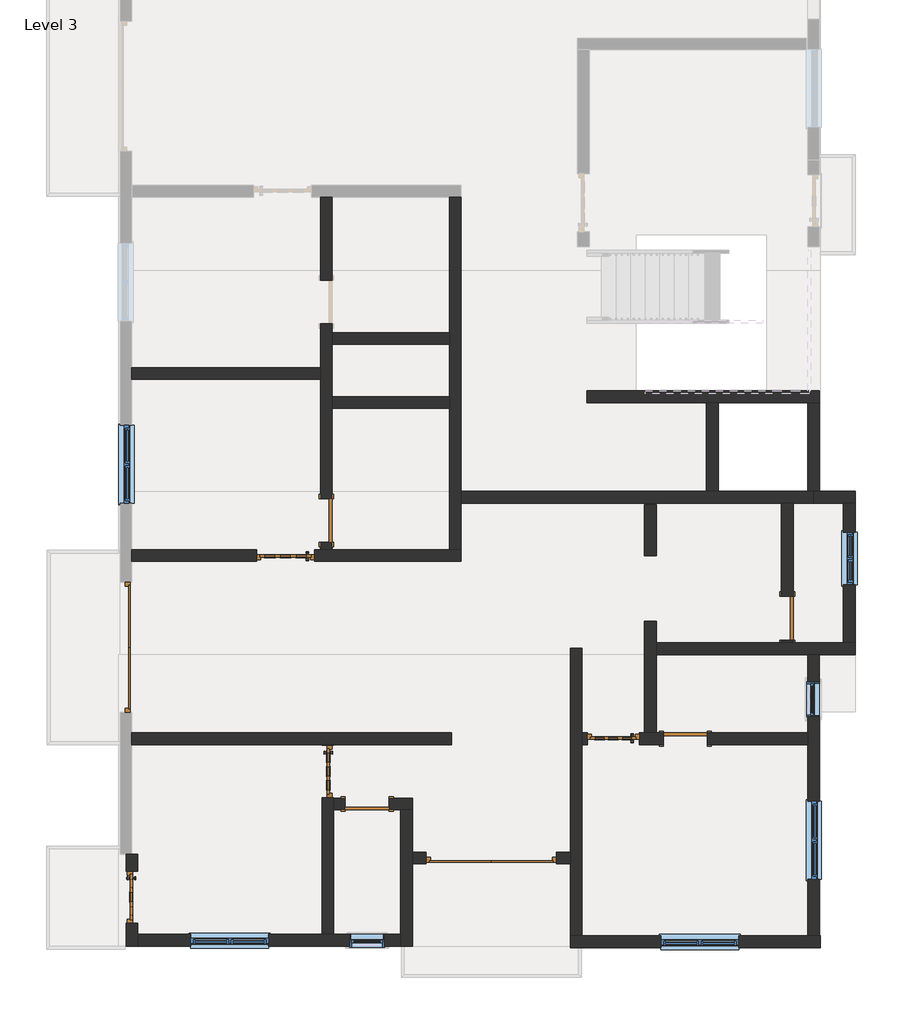
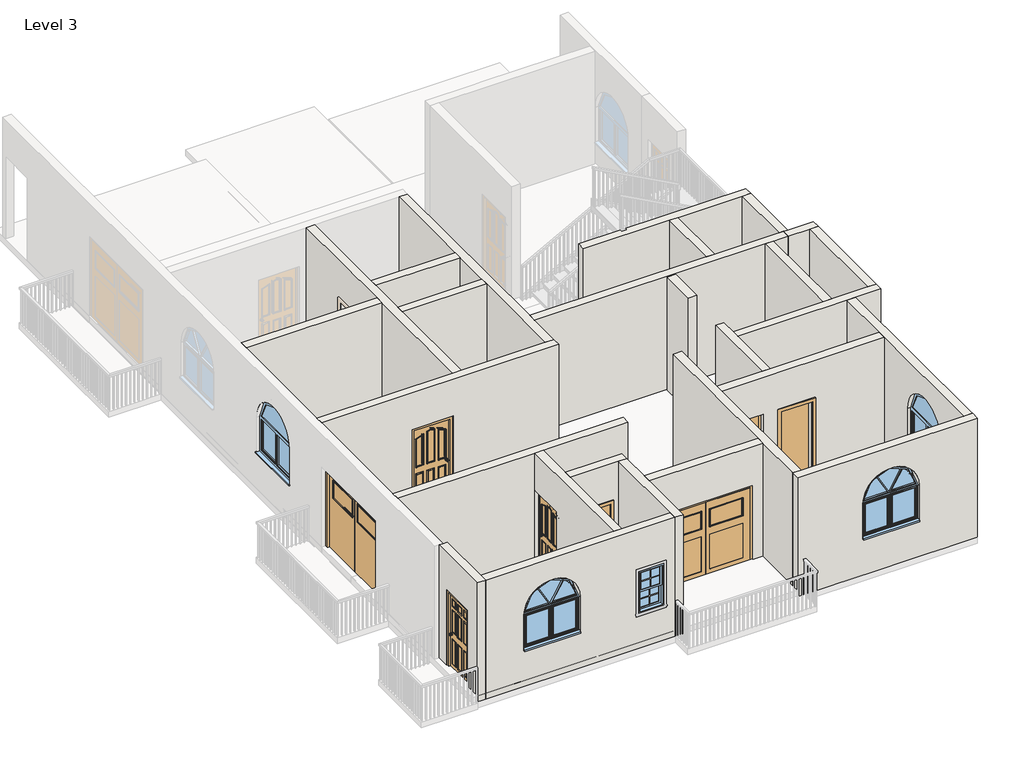
# One storey, part 1 of 7: 27 walls, 10 doors, 7 windows.
# Revit data of these elements (continued)
# Type "Single-Flush : 30\" x 80\"" (continued)
#   Construction Type Id = "MDOOR"
#   Assembly Code = "C1020"
#   Analytic Construction = "Metal"
#   Thickness = 0' - 2"
#   Heat Transfer Coefficient (U) = 0.651978 BTU/(h·ft²·°F)
#   Height = 6' - 8"
#   Trim Projection Ext = 0' - 1"
#   Trim Projection Int = 0' - 1"
#   Trim Width = 0' - 3"
#   Width = 2' - 6"
#   Define Thermal Properties by = 1
#   Define Thermal Properties by = 1
#   Door Material = Door - Panel
#   Frame Material = Door - Frame
#   Visual Light Transmittance = 0
#   Solar Heat Gain Coefficient = 0
#   Function = (empty or 0)
#   Wall Closure = (empty or 0)
# Type "Generic - 9\" w"
#   Assembly Code = "B2010"
#   Layers, outside or top first: 0' - 8" no material (function 1)
# Type "Generic -4.5\" p"
#   Assembly Code = "B2010"
#   Layers, outside or top first: 0' - 8" no material (function 1)
# Type "Window-Double-Hung : 24\" x 42\""
#   Type Mark = "10"
#   Fire Rating = "0.5h"
#   Construction Type Id = "DG-DR"
#   Assembly Code = "B2020100"
#   Analytic Construction = "Double glazing - domestic"
#   Wall Thickness [instance default] = 0' - 6"
#   Window Inset [instance default] = 0' - 0"
#   Visual Light Transmittance = 0.81
#   Thermal Resistance (R) = 1.8146 (h·ft²·°F)/BTU
#   Solar Heat Gain Coefficient = 0.76
#   Muntin Width = 1' - 6"
#   Muntin Height = 1' - 5 1/8"
#   Interior Wall Closure [instance default] = 0' - 1 1/2"
#   Rough Width = 2' - 0 1/2"
#   Rough Height = 3' - 6 1/2"
#   Frame Extension [instance default] = 0' - 1 1/4"
#   Exterior Wall Closure [instance default] = 0' - 0 1/2"
#   Extension Jamb [instance default] = 0' - 1 1/2"
#   Heat Transfer Coefficient (U) = 0.5511 BTU/(h·ft²·°F)
#   Height = 3' - 6"
#   Width = 2' - 0"
#   Define Thermal Properties by = 1
#   Top Muntin Visibility = yes
#   Indicator Visibility [instance default] = yes
#   Extension Jamb Visibility [instance default] = yes
#   Interior Trim Visibility [instance default] = yes
#   Exterior Trim Visibility [instance default] = yes
#   Define Thermal Properties by = 1
#   Bottom Muntin Visibility = yes
#   Muntin Pattern = Muntin Pattern_2x2 : Muntin Pattern_2x2
#   Interior Trim Material = Wood - Stained
#   Interior Trim = Trim-Window-Interior-Flat : Picture Frame
#   Exterior Trim Material = Clad - White
#   Exterior Trim = Trim-Window-Exterior-Flat : with Sill
#   Glass Panel Material = Glass
#   Exterior Frame Material = Clad - White
#   Interior Frame Material = Wood - Stained
#   Wall Closure = (empty or 0)
# Type "Windows_Arched : 1360x910mm"
#   Type Mark = "20"
#   Operation = "UserDefined"
#   Construction Type Id = "GSP4R"
#   Manufacturer = "Revit"
#   Keynote = "L10"
#   Analytic Construction = "1/8 in Pilkington single glazing"
#   Wrap Layers (Ext) from Ext = 0' - 4.03543"
#   Wrap Layers (Int) from Ext = 0' - 6.98819"
#   Window Board Projection = 0' - 0.98425"
#   Window Board Extension = 0' - 0.98425"
#   Visual Light Transmittance = 0.9
#   Solar Heat Gain Coefficient = 0.78
#   Rough Width = 4' - 5.54331"
#   Rough Height = 2' - 11.82677"
#   Height = 2' - 11.82677"
#   Width = 4' - 5.54331"
#   Heat Transfer Coefficient (U) = 0.6496 BTU/(h·ft²·°F)
#   Glazing Thickness = 0' - 0.94488"
#   FrameOffset - External = 0' - 1.9685"
#   Frame Depth = 0' - 2.67717"
#   Default Head Height = 6' - 11.07087"
#   Cill Depth = 0' - 3.44488"
#   Cavity Closer Width = 0' - 1.9685"
#   Cavity Closer Offset from Ext = 0' - 4.03543"
#   Cavity Closer Depth = 0' - 3.34646"
#   Vis - Cavity Closers = yes
#   Define Thermal Properties by = 1
#   Material Trim = Window Frame
#   Material Glass = Glass
#   Material Frame = Window Frame
#   Wall Closure = (empty or 0)
# Type "Windows_Dbl_w-Glazing_Bars : 910x910mm"
#   Type Mark = "33"
#   Operation = "DoublePanelVertical"
#   Construction Type Id = "GSP4R"
#   Manufacturer = "Revit"
#   Keynote = "L10"
#   Analytic Construction = "1/8 in Pilkington single glazing"
#   Wrap Layers (Ext) from Ext = 0' - 4.03543"
#   Wrap Layers (Int) from Ext = 0' - 6.98819"
#   Window Board Projection = 0' - 0.98425"
#   Window Board Extension = 0' - 0.98425"
#   Visual Light Transmittance = 0.9
#   Solar Heat Gain Coefficient = 0.78
#   Rough Width = 2' - 11.82677"
#   Rough Height = 2' - 11.82677"
#   Height = 2' - 11.82677"
#   Width = 2' - 11.82677"
#   Heat Transfer Coefficient (U) = 0.6496 BTU/(h·ft²·°F)
#   Glazing Thickness = 0' - 0.94488"
#   Glazing Bar Thickness = 0' - 0.7874"
#   FrameOffset - External = 0' - 1.9685"
#   Frame Depth = 0' - 2.55906"
#   Default Head Height = 6' - 10.67717"
#   Cill Depth = 0' - 3.44488"
#   Cavity Closer Width = 0' - 1.9685"
#   Cavity Closer Offset from Ext = 0' - 4.03543"
#   Cavity Closer Depth = 0' - 3.34646"
#   Vis - Glazing Bars = yes
#   Vis - Cavity Closers = yes
#   Define Thermal Properties by = 1
#   Material Trim = Window Frame
#   Material Glazing Bars = Window Frame
#   Material Glass = Glass
#   Material Frame = Window Frame
#   Wall Closure = (empty or 0)
# Element 1 (IfcDoor, "Doors_ExtSgl_5 : 910x2110mm")
#   Phase Created = New Construction
#   Materials on its faces: "Door - Panel", "Door - Handle", "Door - Frame/Mullion", "Door - Glazing"
# Element 2 (IfcDoor, "Doors_ExtSgl_6 : 1010x2110mm")
#   Phase Created = New Construction
#   Materials on its faces: "Door - Panel", "Door - Handle", "Door - Frame/Mullion", "Door - Glazing"
# Elements 3, 4 (IfcDoor, "Doors_ExtSgl_6 : 910x2110mm")
#   Phase Created = New Construction
#   Materials on its faces: "Door - Panel", "Door - Handle", "Door - Frame/Mullion", "Door - Glazing"
# Element 5 (IfcDoor, "Doors_Garage_Timber_Side_Hung_Glazing : 2270x2050mm")
#   Phase Created = New Construction
#   Materials on its faces: "Door - Panel", "Door - Frame/Mullion", "Door - Glazing"
# Element 6 (IfcDoor, "Doors_Garage_Timber_Side_Hung_Glazing : 2270x2200mm")
#   Phase Created = New Construction
#   Materials on its faces: "Door - Panel", "Door - Frame/Mullion", "Door - Glazing"
# Elements 7, 8, 9, 10 (IfcDoor, "Single-Flush : 30\" x 80\"")
#   Phase Created = New Construction
#   Materials on its faces: "Door - Frame", "Door - Panel"
# Element 11 (IfcWall, "Generic - 9\" w")
#   Top Offset = 0' - 0"
#   Base Offset = 0' - 0"
#   wall height = 10' - 0"
#   Phase Created = New Construction
#   Base Constraint = Level 3
#   Top Constraint = Level 4
#   Materials on its faces: "Default Wall", "Door - Frame", "Earth"
# Elements 12, 13 (IfcWall, "Generic - 9\" w")
#   Top Offset = 0' - 0"
#   Base Offset = 0' - 0"
#   wall height = 10' - 0"
#   Phase Created = New Construction
#   Base Constraint = Level 3
#   Top Constraint = Level 4
#   Materials on its faces: "Default Wall"
# Element 14 (IfcWall, "Generic - 9\" w")
#   Top Offset = 0' - 0"
#   Base Offset = 0' - 0"
#   wall height = 10' - 0"
#   Phase Created = New Construction
#   Base Constraint = Level 3
#   Top Constraint = Level 4
#   Materials on its faces: "Default Wall", "Door - Frame/Mullion", "Earth"
# Element 15 (IfcWall, "Generic - 9\" w")
#   Top Offset = 0' - 0"
#   Base Offset = 0' - 0"
#   wall height = 10' - 0"
#   Phase Created = New Construction
#   Base Constraint = Level 3
#   Top Constraint = Level 4
#   Materials on its faces: "Default Wall", "Concrete, Lightweight", "Wood - Stained"
# Element 16 (IfcWall, "Generic - 9\" w")
#   Top Offset = 0' - 0"
#   Base Offset = 0' - 0"
#   wall height = 10' - 0"
#   Phase Created = New Construction
#   Base Constraint = Level 3
#   Top Constraint = Level 4
#   Materials on its faces: "Default Wall", "Wood - Stained"
# Element 17 (IfcWall, "Generic - 9\" w")
#   Top Offset = 0' - 0"
#   Base Offset = 0' - 0"
#   wall height = 10' - 0"
#   Phase Created = New Construction
#   Base Constraint = Level 3
#   Top Constraint = Level 4
#   Materials on its faces: "Default Wall", "Earth"
# Elements 18, 19 (IfcWall, "Generic - 9\" w")
#   Top Offset = 0' - 0"
#   Base Offset = 0' - 0"
#   wall height = 10' - 0"
#   Phase Created = New Construction
#   Base Constraint = Level 3
#   Top Constraint = Level 4
#   Materials on its faces: "Default Wall", "Concrete, Lightweight"
# Elements 20, 21, 22, 23, 24, 25, 26, 27, 28, 31, 32, 33, 36, 37 (IfcWall, "Generic -4.5\" p")
#   Top Offset = 0' - 0"
#   Base Offset = 0' - 0"
#   wall height = 10' - 0"
#   Phase Created = New Construction
#   Base Constraint = Level 3
#   Top Constraint = Level 4
#   Materials on its faces: "Default Wall"
# Element 29 (IfcWall, "Generic -4.5\" p")
#   Top Offset = 0' - 0"
#   Base Offset = 0' - 0"
#   wall height = 10' - 0"
#   Phase Created = New Construction
#   Base Constraint = Level 3
#   Top Constraint = Level 4
#   Materials on its faces: "Default Wall", "Concrete, Lightweight"
# Element 30 (IfcWall, "Generic -4.5\" p")
#   Top Offset = 0' - 0"
#   Base Offset = 0' - 0"
#   wall height = 10' - 0"
#   Phase Created = New Construction
#   Base Constraint = Level 3
#   Top Constraint = Level 4
#   Materials on its faces: "Default Wall", "Door - Frame/Mullion"
# Elements 34, 35 (IfcWall, "Generic -4.5\" p")
#   Top Offset = 0' - 0"
#   Base Offset = 0' - 0"
#   wall height = 10' - 0"
#   Phase Created = New Construction
#   Base Constraint = Level 3
#   Top Constraint = Level 4
#   Materials on its faces: "Default Wall", "Earth"
# Element 38 (IfcWindow, "Window-Double-Hung : 24\" x 42\"")
#   Mark = "37"
#   Window Inset = 0' - 0"
#   Interior Wall Closure = 0' - 1 1/2"
#   Frame Extension = 0' - 1 1/4"
#   Exterior Wall Closure = 0' - 0 1/2"
#   Interior Trim Visibility = yes
#   Indicator Visibility = yes
#   Exterior Trim Visibility = yes
#   Phase Created = New Construction
#   Materials on its faces: "Wood - Stained", "Glass", "Clad - White"
# Element 39 (IfcWindow, "Window-Double-Hung : 24\" x 42\"")
#   Mark = "89"
#   Window Inset = 0' - 0"
#   Interior Wall Closure = 0' - 1 1/2"
#   Frame Extension = 0' - 1 1/4"
#   Exterior Wall Closure = 0' - 0 1/2"
#   Interior Trim Visibility = yes
#   Indicator Visibility = yes
#   Exterior Trim Visibility = yes
#   Phase Created = New Construction
#   Materials on its faces: "Wood - Stained", "Glass", "Clad - White"
# Element 40 (IfcWindow, "Windows_Arched : 1360x910mm")
#   Mark = "33"
#   Phase Created = New Construction
#   Materials on its faces: "Window Frame", "Glass"
# Element 41 (IfcWindow, "Windows_Arched : 1360x910mm")
#   Mark = "34"
#   Phase Created = New Construction
#   Materials on its faces: "Window Frame", "Glass"
# Element 42 (IfcWindow, "Windows_Arched : 1360x910mm")
#   Mark = "35"
#   Phase Created = New Construction
#   Materials on its faces: "Window Frame", "Glass"
# Element 43 (IfcWindow, "Windows_Arched : 1360x910mm")
#   Mark = "84"
#   Phase Created = New Construction
#   Materials on its faces: "Window Frame", "Glass"
# Element 44 (IfcWindow, "Windows_Dbl_w-Glazing_Bars : 910x910mm")
#   Mark = "38"
#   Phase Created = New Construction
#   Materials on its faces: "Window Frame", "Glass"
# Materials
#   "Door - Glazing": colour RGB 0 0 255, transparency 0.75
#   "Door - Panel": class "Wood", colour RGB 210 159 95, transparency 0, Cost = 0
#   "Door - Frame/Mullion": class "Wood", colour RGB 212 179 113, transparency 0
#   "Door - Handle": colour RGB 0 0 0, transparency 0
#   "Door - Frame": colour RGB 118 70 51, transparency 0, Cost = 0
#   "Wood - Stained": class "Wood", colour RGB 224 178 126, transparency 0, Cost = 0
#   "Clad - White": class "Wood", colour RGB 242 242 238, transparency 0, Cost = 0
#   "Glass": class "Glass", colour RGB 0 128 192, transparency 0.75, Description = "Soda Lime Glass", Cost = 0
#   "Window Frame": colour RGB 249 249 249, transparency 0
#   "Default Wall": colour RGB 128 128 128, transparency 0, Cost = 0
#   "Earth": class "Generic", colour RGB 97 75 62, transparency 0, Description = "Soil", Cost = 0
#   "Concrete, Lightweight": class "Concrete", colour RGB 142 141 140, transparency 0, Description = "Lightweight concrete", Cost = 0
